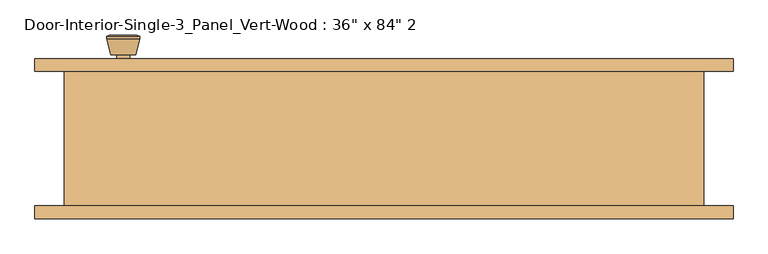
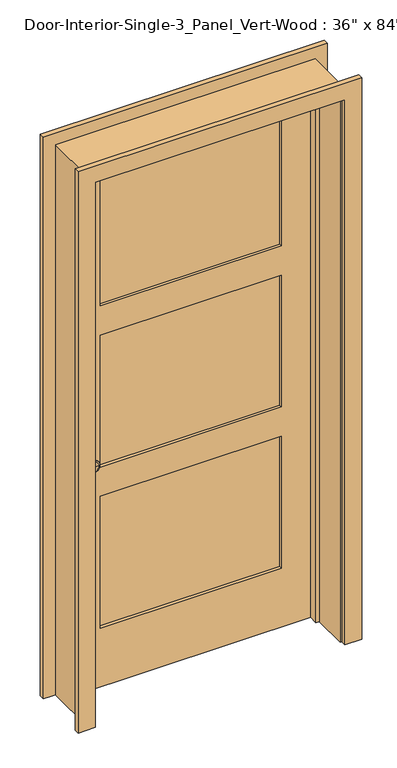
"""IFC4 building model written with IfcOpenShell, lengths in millimetres: door geometry."""

from ifc_helpers import new_model, si_unit, point, frame, frame_2d, origin, place, context, project, spatial, polyline, circle_curve, trimmed, segment, composite_curve, outline, extrude, faceted_brep, source, transform, mapped, element, save
from ifc_brep_helpers import plane_surface, cylinder_surface, revolved_surface, advanced_brep


def door_54d869bf(model_context):
    return source(origin(), model_context, "Body", "SolidModel", [
        advanced_brep(
        [(-393.7, 57.5, 914.4), (-383.7, 57.5, 914.4), (-403.7, 57.5, 914.4), (-373.2241324, 8.5, 914.4), (-393.7, 8.5, 914.4), (-414.1758676, 8.5, 914.4), (-368.7, 10.3278681, 914.4), (-418.7, 10.3278681, 914.4), (-368.7, 13.7915463, 914.4), (-418.7, 13.7915463, 914.4), (-375.063764, 38.5, 914.4), (-412.336236, 38.5, 914.4), (-383.7, 38.5, 914.4), (-403.7, 38.5, 914.4)],
        [
            (0, 1),
            (1, 2, circle_curve(frame((-393.7, 57.5, 914.4), z_axis=(0.0, 1.0, 0.0), x_axis=(-1.0, 0.0, 0.0)), 10.0)),
            (2, 0),
            (2, 1, circle_curve(frame((-393.7, 57.5, 914.4), z_axis=(0.0, 1.0, 0.0), x_axis=(-1.0, 0.0, 0.0)), 10.0)),
            (3, 4),
            (4, 5),
            (5, 3, circle_curve(frame((-393.7, 8.5, 914.4), z_axis=(0.0, -1.0, 0.0), x_axis=(-1.0, 0.0, 0.0)), 20.4758676)),
            (3, 5, circle_curve(frame((-393.7, 8.5, 914.4), z_axis=(0.0, -1.0, 0.0), x_axis=(-1.0, 0.0, 0.0)), 20.4758676)),
            (6, 3),
            (5, 7),
            (7, 6, circle_curve(frame((-393.7, 10.3278681, 914.4), z_axis=(0.0, -1.0, 0.0), x_axis=(-1.0, 0.0, 0.0)), 25.0)),
            (6, 7, circle_curve(frame((-393.7, 10.3278681, 914.4), z_axis=(0.0, -1.0, 0.0), x_axis=(-1.0, 0.0, 0.0)), 25.0)),
            (8, 6),
            (7, 9),
            (9, 8, circle_curve(frame((-393.7, 13.7915463, 914.4), z_axis=(0.0, -1.0, 0.0), x_axis=(-1.0, 0.0, 0.0)), 25.0)),
            (8, 9, circle_curve(frame((-393.7, 13.7915463, 914.4), z_axis=(0.0, -1.0, 0.0), x_axis=(-1.0, 0.0, 0.0)), 25.0)),
            (10, 8),
            (9, 11),
            (11, 10, circle_curve(frame((-393.7, 38.5, 914.4), z_axis=(0.0, -1.0, 0.0), x_axis=(-1.0, 0.0, 0.0)), 18.636236)),
            (10, 11, circle_curve(frame((-393.7, 38.5, 914.4), z_axis=(0.0, -1.0, 0.0), x_axis=(-1.0, 0.0, 0.0)), 18.636236)),
            (12, 10),
            (11, 13),
            (13, 12, circle_curve(frame((-393.7, 38.5, 914.4), z_axis=(0.0, -1.0, 0.0), x_axis=(-1.0, 0.0, 0.0)), 10.0)),
            (12, 13, circle_curve(frame((-393.7, 38.5, 914.4), z_axis=(0.0, -1.0, 0.0), x_axis=(-1.0, 0.0, 0.0)), 10.0)),
            (1, 12),
            (13, 2),
        ],
        [
            plane_surface(frame((-393.7, 57.5, 914.4), z_axis=(0.0, 1.0, 0.0), x_axis=(-1.0, 0.0, 0.0))),
            plane_surface(frame((-393.7, 8.5, 914.4), z_axis=(0.0, -1.0, 0.0), x_axis=(-1.0, 0.0, 0.0))),
            revolved_surface(polyline([(-414.1758676, 8.5, 914.4), (-418.7, 10.3278681, 914.4)]), (-393.7, 57.5, 914.4), (0.0, 1.0, 0.0)),
            cylinder_surface(frame((-393.7, 57.5, 914.4), z_axis=(0.0, 1.0, 0.0), x_axis=(-1.0, 0.0, 0.0)), 25.0),
            revolved_surface(polyline([(-418.7, 13.7915463, 914.4), (-412.336236, 38.5, 914.4)]), (-393.7, 57.5, 914.4), (0.0, 1.0, 0.0)),
            plane_surface(frame((-393.7, 38.5, 914.4), z_axis=(0.0, 1.0, 0.0), x_axis=(-1.0, 0.0, 0.0))),
            cylinder_surface(frame((-393.7, 57.5, 914.4), z_axis=(0.0, 1.0, 0.0), x_axis=(-1.0, 0.0, 0.0)), 10.0),
        ],
        [
            (0, [[1, 2, 3]]),
            (0, [[-3, 4, -1]]),
            (1, [[5, 6, 7]]),
            (1, [[-6, -5, 8]]),
            (2, [[9, -7, 10, 11]]),
            (2, [[-10, -8, -9, 12]]),
            (3, [[13, -11, 14, 15]]),
            (3, [[-14, -12, -13, 16]]),
            (4, [[17, -15, 18, 19]]),
            (4, [[-18, -16, -17, 20]]),
            (5, [[21, -19, 22, 23]]),
            (5, [[-22, -20, -21, 24]]),
            (6, [[25, -23, 26, -2]]),
            (6, [[-26, -24, -25, -4]]),
        ],
    ),
        extrude(outline(composite_curve([segment(trimmed(circle_curve(frame_2d((914.4, -393.7)), 30.0), [point((914.4, -423.7))], [point((914.4, -363.7))], False, "CARTESIAN"), True, "CONTINUOUS"), segment(trimmed(circle_curve(frame_2d((914.4, -393.7)), 30.0), [point((914.4, -363.7))], [point((914.4, -423.7))], False, "CARTESIAN"), True, "CONTINUOUS")], self_intersect=False)), frame((0.0, 57.5, 0.0), z_axis=(0.0, 1.0, 0.0), x_axis=(0.0, 0.0, 1.0)), (0.0, 0.0, 1.0), 6.0),
        advanced_brep(
        [(-393.7, 104.425, 914.4), (-403.7, 104.425, 914.4), (-383.7, 104.425, 914.4), (-373.2241324, 153.425, 914.4), (-414.1758676, 153.425, 914.4), (-393.7, 153.425, 914.4), (-368.7, 151.5971319, 914.4), (-418.7, 151.5971319, 914.4), (-368.7, 148.1334537, 914.4), (-418.7, 148.1334537, 914.4), (-375.063764, 123.425, 914.4), (-412.336236, 123.425, 914.4), (-383.7, 123.425, 914.4), (-403.7, 123.425, 914.4)],
        [
            (0, 1),
            (1, 2, circle_curve(frame((-393.7, 104.425, 914.4), z_axis=(0.0, -1.0, 0.0), x_axis=(-1.0, 0.0, 0.0)), 10.0)),
            (2, 0),
            (2, 1, circle_curve(frame((-393.7, 104.425, 914.4), z_axis=(0.0, -1.0, 0.0), x_axis=(-1.0, 0.0, 0.0)), 10.0)),
            (3, 4, circle_curve(frame((-393.7, 153.425, 914.4), z_axis=(0.0, 1.0, 0.0), x_axis=(-1.0, 0.0, 0.0)), 20.4758676)),
            (4, 5),
            (5, 3),
            (4, 3, circle_curve(frame((-393.7, 153.425, 914.4), z_axis=(0.0, 1.0, 0.0), x_axis=(-1.0, 0.0, 0.0)), 20.4758676)),
            (6, 7, circle_curve(frame((-393.7, 151.5971319, 914.4), z_axis=(0.0, 1.0, 0.0), x_axis=(-1.0, 0.0, 0.0)), 25.0)),
            (7, 4),
            (3, 6),
            (7, 6, circle_curve(frame((-393.7, 151.5971319, 914.4), z_axis=(0.0, 1.0, 0.0), x_axis=(-1.0, 0.0, 0.0)), 25.0)),
            (8, 9, circle_curve(frame((-393.7, 148.1334537, 914.4), z_axis=(0.0, 1.0, 0.0), x_axis=(-1.0, 0.0, 0.0)), 25.0)),
            (9, 7),
            (6, 8),
            (9, 8, circle_curve(frame((-393.7, 148.1334537, 914.4), z_axis=(0.0, 1.0, 0.0), x_axis=(-1.0, 0.0, 0.0)), 25.0)),
            (10, 11, circle_curve(frame((-393.7, 123.425, 914.4), z_axis=(0.0, 1.0, 0.0), x_axis=(-1.0, 0.0, 0.0)), 18.636236)),
            (11, 9),
            (8, 10),
            (11, 10, circle_curve(frame((-393.7, 123.425, 914.4), z_axis=(0.0, 1.0, 0.0), x_axis=(-1.0, 0.0, 0.0)), 18.636236)),
            (12, 13, circle_curve(frame((-393.7, 123.425, 914.4), z_axis=(0.0, 1.0, 0.0), x_axis=(-1.0, 0.0, 0.0)), 10.0)),
            (13, 11),
            (10, 12),
            (13, 12, circle_curve(frame((-393.7, 123.425, 914.4), z_axis=(0.0, 1.0, 0.0), x_axis=(-1.0, 0.0, 0.0)), 10.0)),
            (1, 13),
            (12, 2),
        ],
        [
            plane_surface(frame((-393.7, 104.425, 914.4), z_axis=(0.0, -1.0, 0.0), x_axis=(-1.0, 0.0, 0.0))),
            plane_surface(frame((-393.7, 153.425, 914.4), z_axis=(0.0, 1.0, 0.0), x_axis=(-1.0, 0.0, 0.0))),
            revolved_surface(polyline([(-414.1758676, 153.425, 914.4), (-418.7, 151.5971319, 914.4)]), (-393.7, 104.425, 914.4), (0.0, -1.0, 0.0)),
            cylinder_surface(frame((-393.7, 104.425, 914.4), z_axis=(0.0, -1.0, 0.0), x_axis=(-1.0, 0.0, 0.0)), 25.0),
            revolved_surface(polyline([(-418.7, 148.1334537, 914.4), (-412.336236, 123.425, 914.4)]), (-393.7, 104.425, 914.4), (0.0, -1.0, 0.0)),
            plane_surface(frame((-393.7, 123.425, 914.4), z_axis=(0.0, -1.0, 0.0), x_axis=(-1.0, 0.0, 0.0))),
            cylinder_surface(frame((-393.7, 104.425, 914.4), z_axis=(0.0, -1.0, 0.0), x_axis=(-1.0, 0.0, 0.0)), 10.0),
        ],
        [
            (0, [[1, 2, 3]]),
            (0, [[-3, 4, -1]]),
            (1, [[5, 6, 7]]),
            (1, [[8, -7, -6]]),
            (2, [[9, 10, -5, 11]]),
            (2, [[12, -11, -8, -10]]),
            (3, [[13, 14, -9, 15]]),
            (3, [[16, -15, -12, -14]]),
            (4, [[17, 18, -13, 19]]),
            (4, [[20, -19, -16, -18]]),
            (5, [[21, 22, -17, 23]]),
            (5, [[24, -23, -20, -22]]),
            (6, [[-2, 25, -21, 26]]),
            (6, [[-4, -26, -24, -25]]),
        ],
    ),
        extrude(outline(composite_curve([segment(trimmed(circle_curve(frame_2d((914.4, -393.7)), 30.0), [point((914.4, -423.7))], [point((914.4, -363.7))], False, "CARTESIAN"), True, "CONTINUOUS"), segment(trimmed(circle_curve(frame_2d((914.4, -393.7)), 30.0), [point((914.4, -363.7))], [point((914.4, -423.7))], False, "CARTESIAN"), True, "CONTINUOUS")], self_intersect=False)), frame((0.0, 98.425, 0.0), z_axis=(0.0, 1.0, 0.0), x_axis=(0.0, 0.0, 1.0)), (0.0, 0.0, 1.0), 6.0),
        extrude(outline(polyline([(336.55, 75.1416667), (-336.55, 75.1416667), (-336.55, 86.7833333), (336.55, 86.7833333), (336.55, 75.1416667)])), frame((0.0, 0.0, 1496.4833333), z_axis=(0.0, 0.0, 1.0), x_axis=(1.0, 0.0, 0.0)), (0.0, 0.0, 1.0), 518.0541667),
        extrude(outline(polyline([(336.55, 75.1416667), (-336.55, 75.1416667), (-336.55, 86.7833333), (336.55, 86.7833333), (336.55, 75.1416667)])), frame((0.0, 0.0, 231.775), z_axis=(0.0, 0.0, 1.0), x_axis=(1.0, 0.0, 0.0)), (0.0, 0.0, 1.0), 518.0541667),
        extrude(outline(polyline([(336.55, 75.1416667), (-336.55, 75.1416667), (-336.55, 86.7833333), (336.55, 86.7833333), (336.55, 75.1416667)])), frame((0.0, 0.0, 864.1291667), z_axis=(0.0, 0.0, 1.0), x_axis=(1.0, 0.0, 0.0)), (0.0, 0.0, 1.0), 518.0541667),
        extrude(outline(polyline([(2133.6, -457.2), (0.0, -457.2), (0.0, 457.2), (2133.6, 457.2), (2133.6, -457.2)]), holes=[polyline([(2014.5375, -336.55), (2014.5375, 336.55), (1496.4833333, 336.55), (1496.4833333, -336.55), (2014.5375, -336.55)]), polyline([(749.8291667, -336.55), (749.8291667, 336.55), (231.775, 336.55), (231.775, -336.55), (749.8291667, -336.55)]), polyline([(1382.1833333, -336.55), (1382.1833333, 336.55), (864.1291667, 336.55), (864.1291667, -336.55), (1382.1833333, -336.55)])]), frame((0.0, 63.5, 0.0), z_axis=(0.0, 1.0, 0.0), x_axis=(0.0, 0.0, 1.0)), (0.0, 0.0, 1.0), 34.925),
        faceted_brep([(482.6, 98.425, 0.0), (482.6, -104.775, 0.0), (457.2, -104.775, 0.0), (457.2, 28.575, 0.0), (444.5, 28.575, 0.0), (444.5, 63.5, 0.0), (457.2, 63.5, 0.0), (457.2, 98.425, 0.0), (482.6, 98.425, 2159.0), (482.6, -104.775, 2159.0), (-482.6, -104.775, 2159.0), (-482.6, -104.775, 0.0), (-457.2, -104.775, 0.0), (-457.2, -104.775, 2133.6), (457.2, -104.775, 2133.6), (457.2, 28.575, 2133.6), (-457.2, 28.575, 2133.6), (-457.2, 28.575, 0.0), (-444.5, 28.575, 0.0), (-444.5, 28.575, 2120.9), (444.5, 28.575, 2120.9), (444.5, 63.5, 2120.9), (-444.5, 63.5, 2120.9), (-444.5, 63.5, 0.0), (-457.2, 63.5, 0.0), (-457.2, 63.5, 2133.6), (457.2, 63.5, 2133.6), (457.2, 98.425, 2133.6), (-457.2, 98.425, 2133.6), (-457.2, 98.425, 0.0), (-482.6, 98.425, 0.0), (-482.6, 98.425, 2159.0)], [[[0, 1, 2, 3, 4, 5, 6, 7]], [[1, 0, 8, 9]], [[2, 1, 9, 10, 11, 12, 13, 14]], [[3, 2, 14, 15]], [[4, 3, 15, 16, 17, 18, 19, 20]], [[5, 4, 20, 21]], [[6, 5, 21, 22, 23, 24, 25, 26]], [[7, 6, 26, 27]], [[0, 7, 27, 28, 29, 30, 31, 8]], [[9, 8, 31, 10]], [[15, 14, 13, 16]], [[21, 20, 19, 22]], [[27, 26, 25, 28]], [[30, 29, 24, 23, 18, 17, 12, 11]], [[10, 31, 30, 11]], [[16, 13, 12, 17]], [[22, 19, 18, 23]], [[28, 25, 24, 29]]]),
        extrude(outline(polyline([(0.0, 463.55), (0.0, 527.05), (2203.45, 527.05), (2203.45, -527.05), (0.0, -527.05), (0.0, -463.55), (2139.95, -463.55), (2139.95, 463.55), (0.0, 463.55)])), frame((0.0, -123.825, 0.0), z_axis=(0.0, 1.0, 0.0), x_axis=(0.0, 0.0, 1.0)), (0.0, 0.0, 1.0), 19.05),
        extrude(outline(polyline([(0.0, 463.55), (0.0, 527.05), (2203.45, 527.05), (2203.45, -527.05), (0.0, -527.05), (0.0, -463.55), (2139.95, -463.55), (2139.95, 463.55), (0.0, 463.55)])), frame((0.0, 98.425, 0.0), z_axis=(0.0, 1.0, 0.0), x_axis=(0.0, 0.0, 1.0)), (0.0, 0.0, 1.0), 19.05),
    ])


if __name__ == "__main__":
    model = new_model("IFC4")
    model_context = context("Model", 3, world=origin())
    ifc_project = project(units=[si_unit("LENGTHUNIT", "METRE", prefix="MILLI")], contexts=[model_context])
    site = spatial("IfcSite", under=ifc_project)
    building = spatial("IfcBuilding", under=site)
    placement = place(None, origin())
    door_shape = door_54d869bf(model_context)
    element("IfcDoor", 1, ObjectType="Door-Interior-Single-3_Panel_Vert-Wood : 36\" x 84\" 2", at=placement, inside=building, context=model_context, shape_type="MappedRepresentation", body=[
        mapped(door_shape, transform((0.0, 0.0, 0.0), x_axis=(1.0, 0.0, 0.0), y_axis=(0.0, 1.0, 0.0), z_axis=(0.0, 0.0, 1.0))),
    ])
    save(model, "model.ifc")

# Revit data of these elements
# Type "Door-Interior-Single-3_Panel_Vert-Wood : 36\" x 84\" 2"
#   Type Mark = "11"
#   Assembly Code = "C1020300"
#   Analytic Construction = "Wooden"
#   Top Rail = 0' - 4 11/16"
#   Thickness = 0' - 1 3/8"
#   Thermal Resistance (R) = 2.5876 (h·ft²·°F)/BTU
#   Swing Angle [instance default] = 90.00°
#   Stiles = 0' - 4 3/4"
#   Rough Width = 3' - 2"
#   Rough Height = 7' - 1"
#   Intermediate Rail = 0' - 4 1/2"
#   Height = 7' - 0"
#   Width = 3' - 0"
#   Heat Transfer Coefficient (U) = 0.3865 BTU/(h·ft²·°F)
#   Bottom Rail = 0' - 9 1/8"
#   Trim Material = Cherry
#   Panel Material = Door - Panel
#   Frame Material = Door - Panel
#   Door Handle Material = Aluminum
#   Visual Light Transmittance = 0
#   Solar Heat Gain Coefficient = 0
#   Wall Closure = (empty or 0)
#   Function = (empty or 0)
# Element 1 (IfcDoor, "Door-Interior-Single-3_Panel_Vert-Wood : 36\" x 84\" 2")
#   Materials on its faces: "Door - Panel", "Aluminum", "Cherry"
# Materials
#   "Cherry": class "Wood", colour RGB 226 177 128, transparency 0, Description = "Prunus Serotina", Cost = 0
#   "Door - Panel": class "Wood", colour RGB 210 159 95, transparency 0
#   "Aluminum": class "Metal", colour RGB 247 247 247, transparency 0, Description = "Aluminum 6061", Cost = 0
